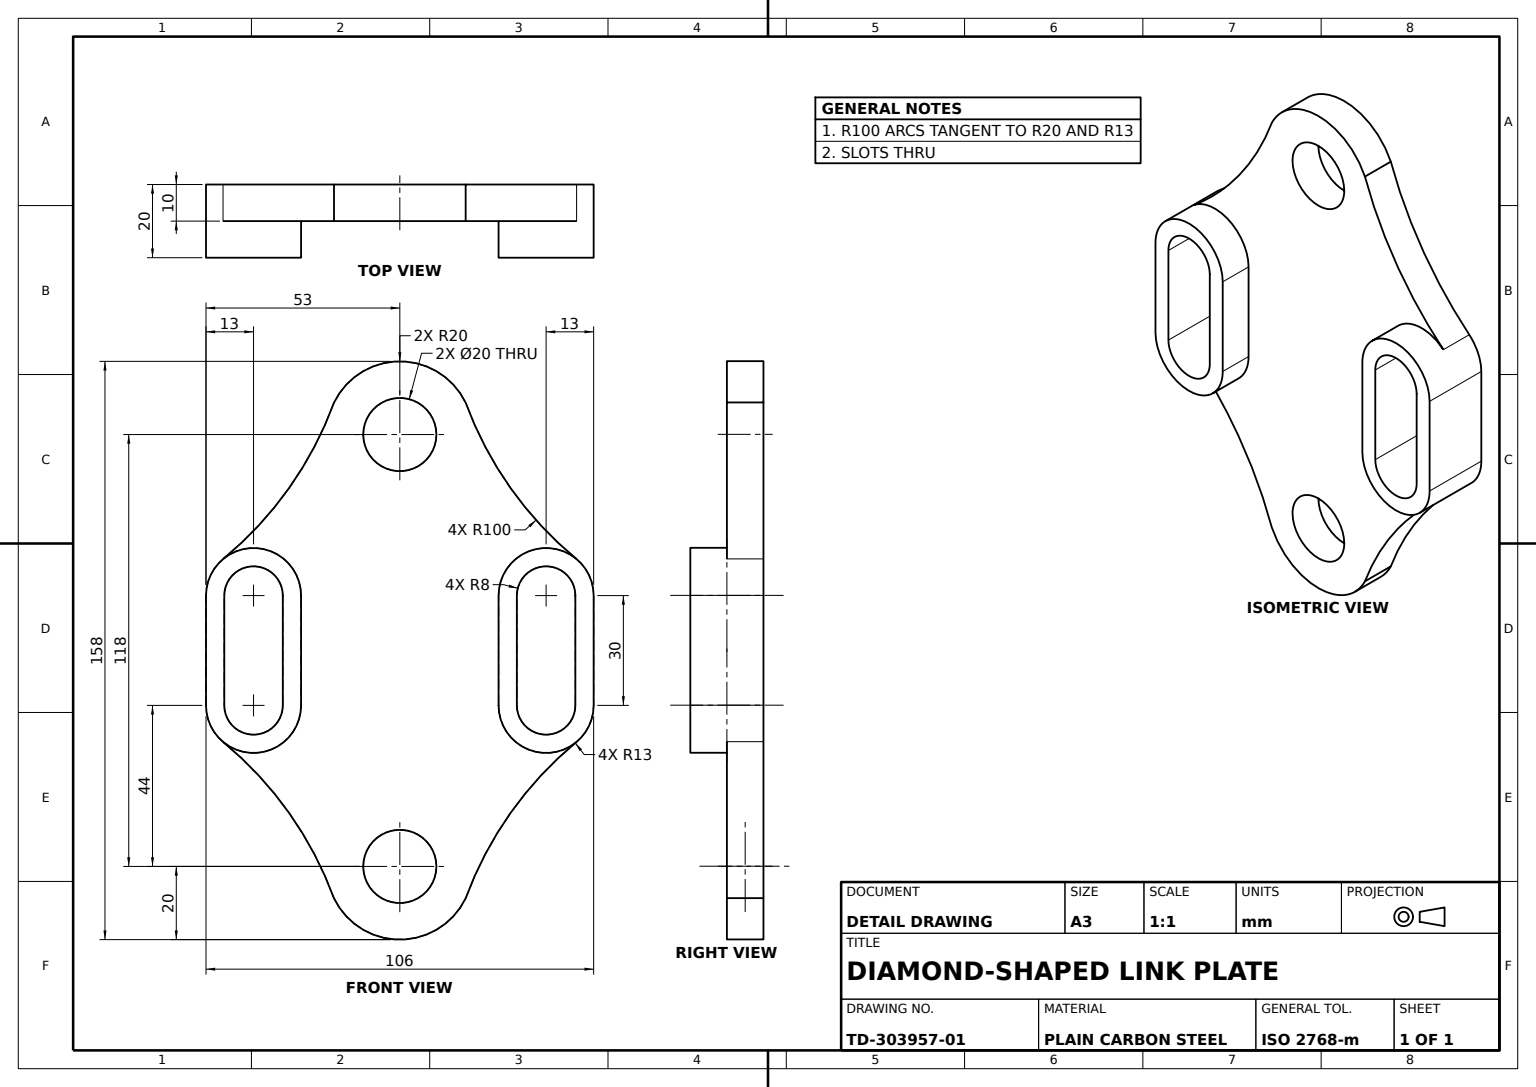
from build123d import *

# Parameters (mm, degrees)
DIAMOND_PLATE_DEPTH    = 10
THROUGH_SLOTS_2X_DEPTH = 10
SLOT_BOSS_A_DEPTH      = 10
END_HOLES_PROFILE_R    = 10
END_HOLES_2X_DEPTH     = 10
SLOT_BOSS_B_DEPTH      = 10


with BuildPart() as part:
    # Diamond Plate Profile → Diamond Plate (new body)
    with BuildSketch(Plane.XY):
        with BuildLine():
            ThreePointArc((48.341000131, -83.971344784), (51.777796944, -79.503044534), (53, -74))
            Line((53, -74), (53, -44))
            ThreePointArc((53, -44), (51.777796944, -38.496955466), (48.341000131, -34.028655216))
            ThreePointArc((48.341000131, -34.028655216), (30.319444036, -14.678569552), (17.999640508, 8.718540106))
            ThreePointArc((17.999640508, 8.718540106), (0, 20), (-17.999640508, 8.718540106))
            ThreePointArc((-17.999640508, 8.718540106), (-30.319444036, -14.678569552), (-48.341000131, -34.028655216))
            ThreePointArc((-48.341000131, -34.028655216), (-51.777796944, -38.496955466), (-53, -44))
            Line((-53, -44), (-53, -74))
            ThreePointArc((-53, -74), (-51.777796944, -79.503044534), (-48.341000131, -83.971344784))
            ThreePointArc((-48.341000131, -83.971344784), (-48.2675462, -84.031821869), (-48.194149845, -84.092368816))
            ThreePointArc((-48.194149845, -84.092368816), (-30.264409293, -103.399045748), (-17.999640508, -126.718540106))
            ThreePointArc((-17.999640508, -126.718540106), (0, -138), (17.999640508, -126.718540106))
            ThreePointArc((17.999640508, -126.718540106), (30.319444036, -103.321430448), (48.341000131, -83.971344784))
        make_face()
    extrude(amount=DIAMOND_PLATE_DEPTH)

    # Slot Cuts Profile → Through Slots 2x (cut)
    with BuildSketch(Plane.XY.offset(10)):
        with BuildLine():
            Line((-47.999999999, -44), (-47.999999999, -74))
            ThreePointArc((-47.999999999, -74), (-40, -81.999999999), (-32, -74))
            Line((-32, -74), (-32, -44))
            ThreePointArc((-32, -44), (-40, -36.000000001), (-47.999999999, -44))
        make_face()
        with BuildLine():
            Line((32, -44), (32, -74))
            ThreePointArc((32, -74), (40, -81.999999999), (47.999999999, -74))
            Line((47.999999999, -74), (47.999999999, -44))
            ThreePointArc((47.999999999, -44), (40, -36.000000001), (32, -44))
        make_face()
    extrude(amount=-THROUGH_SLOTS_2X_DEPTH, mode=Mode.SUBTRACT)

    # Slot Boss A Profile → Slot Boss A (add)
    with BuildSketch(Plane.XY.offset(10)):
        with BuildLine():
            Line((-27, -44), (-27, -74))
            ThreePointArc((-27, -74), (-40, -87), (-53, -74))
            Line((-53, -74), (-53, -44))
            ThreePointArc((-53, -44), (-40, -31), (-27, -44))
        make_face()
        with BuildLine():
            Line((-32, -44), (-32, -74))
            ThreePointArc((-32, -74), (-40, -81.999999999), (-47.999999999, -74))
            Line((-47.999999999, -74), (-47.999999999, -44))
            ThreePointArc((-47.999999999, -44), (-40, -36.000000001), (-32, -44))
        make_face(mode=Mode.SUBTRACT)
    extrude(amount=SLOT_BOSS_A_DEPTH)

    # End Holes Profile → End Holes 2x (cut)
    with BuildSketch(Plane.XY.offset(10)):
        Circle(END_HOLES_PROFILE_R)
        with Locations((0, -118)):
            Circle(END_HOLES_PROFILE_R)
    extrude(amount=-END_HOLES_2X_DEPTH, mode=Mode.SUBTRACT)

    # Slot Boss B Profile → Slot Boss B (add)
    with BuildSketch(Plane.XY.offset(10)):
        with BuildLine():
            Line((27, -44), (27, -74))
            ThreePointArc((27, -74), (40, -87), (53, -74))
            Line((53, -74), (53, -44))
            ThreePointArc((53, -44), (40, -31), (27, -44))
        make_face()
        with BuildLine():
            Line((32, -44), (32, -74))
            ThreePointArc((32, -74), (40, -81.999999999), (47.999999999, -74))
            Line((47.999999999, -74), (47.999999999, -44))
            ThreePointArc((47.999999999, -44), (40, -36.000000001), (32, -44))
        make_face(mode=Mode.SUBTRACT)
    extrude(amount=SLOT_BOSS_B_DEPTH)


solid = part.part
